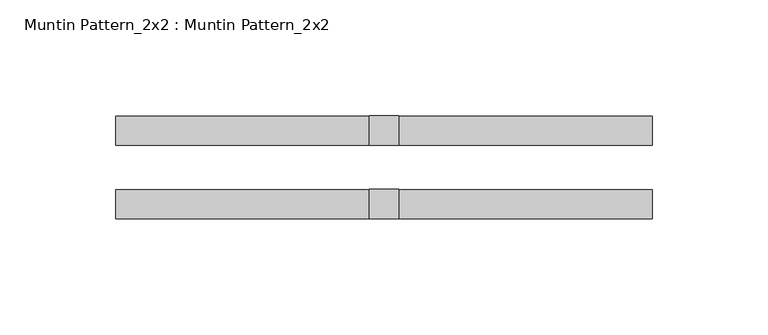
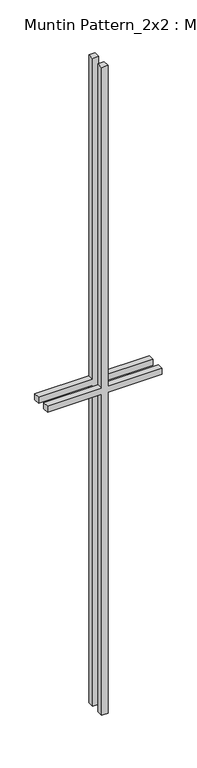
"""IFC4 building model written with IfcOpenShell, lengths in millimetres: proxy geometry, Muntin Pattern_2x2 : Muntin Pattern_2x2."""

from ifc_helpers import new_model, si_unit, frame, origin, place, context, project, spatial, polyline, outline, extrude, source, transform, mapped, element, save


def muntin_pattern_2x2_muntin_pattern_2x2_5c299dc3(model_context):
    return source(origin(), model_context, "Body", "SweptSolid", [
        extrude(outline(polyline([(698.5, -6.35), (698.5, -115.8875), (685.8, -115.8875), (685.8, -6.35), (0.0, -6.35), (0.0, 6.35), (685.8, 6.35), (685.8, 115.8875), (698.5, 115.8875), (698.5, 6.35), (1384.3, 6.35), (1384.3, -6.35), (698.5, -6.35)])), frame((0.0, -22.225, 0.0), z_axis=(0.0, 1.0, 0.0), x_axis=(0.0, 0.0, 1.0)), (0.0, 0.0, 1.0), 12.7),
        extrude(outline(polyline([(698.5, -6.35), (698.5, -115.8875), (685.8, -115.8875), (685.8, -6.35), (0.0, -6.35), (0.0, 6.35), (685.8, 6.35), (685.8, 115.8875), (698.5, 115.8875), (698.5, 6.35), (1384.3, 6.35), (1384.3, -6.35), (698.5, -6.35)])), frame((0.0, 9.525, 0.0), z_axis=(0.0, 1.0, 0.0), x_axis=(0.0, 0.0, 1.0)), (0.0, 0.0, 1.0), 12.7),
    ])


if __name__ == "__main__":
    model = new_model("IFC4")
    model_context = context("Model", 3, world=origin())
    ifc_project = project(units=[si_unit("LENGTHUNIT", "METRE", prefix="MILLI")], contexts=[model_context])
    site = spatial("IfcSite", under=ifc_project)
    building = spatial("IfcBuilding", under=site)
    placement = place(None, origin())
    muntin_pattern_2x2_muntin_pattern_2x2_shape = muntin_pattern_2x2_muntin_pattern_2x2_5c299dc3(model_context)
    element("IfcBuildingElementProxy", 1, Name="Muntin Pattern_2x2 : Muntin Pattern_2x2", ObjectType="Muntin Pattern_2x2 : Muntin Pattern_2x2", at=placement, inside=building, context=model_context, shape_type="MappedRepresentation", body=[
        mapped(muntin_pattern_2x2_muntin_pattern_2x2_shape, transform((0.0, 0.0, 0.0), x_axis=(1.0, 0.0, 0.0), y_axis=(0.0, 1.0, 0.0), z_axis=(0.0, 0.0, 1.0))),
    ])
    save(model, "model.ifc")

# Revit data of these elements
# Type "Muntin Pattern_2x2 : Muntin Pattern_2x2"
#   Width [instance default] = 4' - 0"
#   Thickness = 0' - 0 1/2"
#   Height [instance default] = 4' - 0"
#   Distance = 0' - 0 3/4"
#   Interior Material [instance default] = none
#   Exterior Material [instance default] = none
#   Default Elevation = 0
# Element 1 (IfcBuildingElementProxy, "Muntin Pattern_2x2 : Muntin Pattern_2x2")
#   Width = 0' - 9 1/8"
#   Height = 4' - 6 1/2"
#   Interior Material = Wood - Stained
#   Exterior Material = Clad - White
#   Materials on its faces: "Clad - White", "Wood - Stained"
# Materials
#   "Clad - White": class "Wood", colour RGB 242 242 238, transparency 0, Cost = 0
#   "Wood - Stained": class "Wood", colour RGB 224 178 126, transparency 0, Cost = 0
